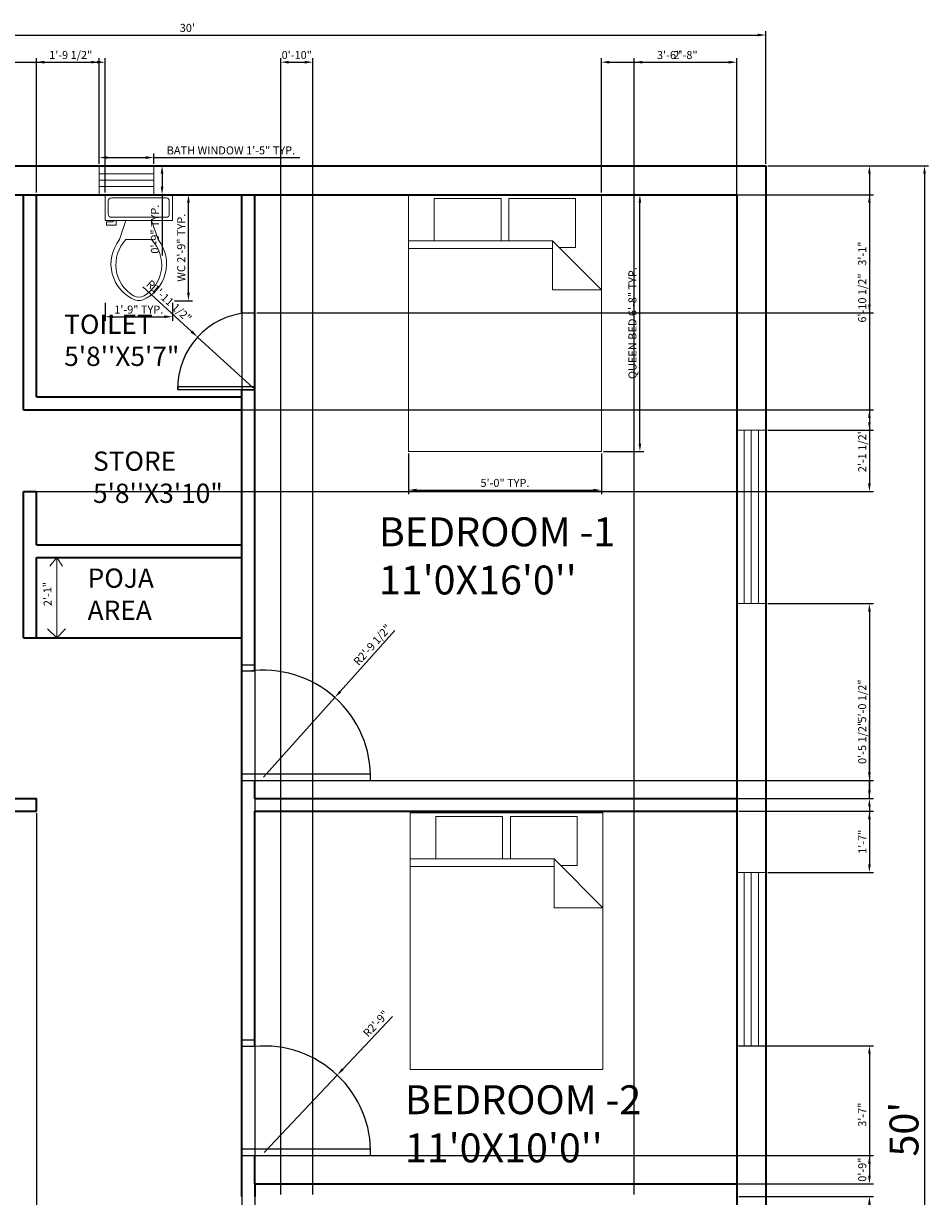
# Model space of a CAD drawing. Units: inches. Extents: x 2572 to 3021, y 1553 to 2232.
# Tile 3 of 3: x 2739 to 3021, y 1866 to 2232. Entities that reach past the tile are written whole.
import ezdxf

# ---------------------------------------------------------------- set-up
doc = ezdxf.new("R2010")
doc.units = ezdxf.units.IN
for name, color, linetype, lineweight in [('A-ANNO-DIMS', 2, 'Continuous', 18), ('A-AREA-IDEN', 7, 'Continuous', 25), ('A-DOOR', 3, 'Continuous', 25), ('A-FLOR-FIXT', 9, 'Continuous', 18), ('A-FURN', 8, 'Continuous', 18), ('A-GLAZ', 4, 'Continuous', 18), ('A-WALL', 7, 'Continuous', 35)]:
    doc.layers.add(name, color=color, linetype=linetype, lineweight=lineweight)
doc.styles.get("Standard").update_dxf_attribs({"font": 'arial.ttf'})
doc.dimstyles.new('ISO-25', dxfattribs={"dimtxt": 2.5, "dimasz": 2.5, "dimexe": 1.25, "dimexo": 0.625, "dimtad": 1, "dimdec": 1, "dimlunit": 3, "dimtxsty": 'Standard', "dimcen": 2.5, "dimadec": 0, "dimazin": 0, "dimtfac": 1, "dimtdec": 1, "dimtmove": 0, "dimatfit": 3, "dimfxl": 1, "dimarcsym": 0})

# ---------------------------------------------------------------- blocks, each defined once
blk = doc.blocks.new('Bed - Queen')
for p, q in [((0, -80.00003), (0, 0)), ((0, 0), (59.99999, 0)), ((59.99999, 0), (59.99999, -80.00003)), ((7.99999, -1.2), (28.79998, -1.2)), ((7.99999, -14.4), (7.99999, -1.2)), ((28.79998, -1.2), (28.79998, -14.4)), ((31.19999, -1.2), (51.99999, -1.2)), ((31.19999, -14.4), (31.19999, -1.2)), ((51.99999, -1.2), (51.99999, -16.4)), ((0, -14.4), (44.8, -14.4)), ((59.99999, -29.6), (44.8, -14.4)), ((44.8, -14.4), (44.8, -29.6)), ((44.8, -16.8), (0, -16.8)), ((51.99999, -16.4), (46.79936, -16.4)), ((44.8, -29.6), (59.99999, -29.6)), ((59.99999, -80.00003), (0, -80.00003))]:
    blk.add_line(p, q)
blk = doc.blocks.new('Toilet - top')
for p, q in [((9.5, -6), (9.5, -2)), ((-10, -8.5), (-8, -8.5)), ((-10, -9.5), (-10, -8.5)), ((-7, -9.5), (-10, -9.5)), ((-8, -8.5), (-8, -8)), ((-7, -8), (-7, -9.5)), ((-4, -8), (-6, -14)), ((4, -8), (6, -14)), ((4, -14), (-4, -14))]:
    blk.add_line(p, q)
blk.add_lwpolyline([(10.5, -8), (10.5, 0), (-10.5, 0), (-10.5, -8)], close=True)
for points in [[(-9.5, -2), (-9.5, -6)], [(8.5, -1), (-8.5, -1)], [(-8.5, -7), (8.5, -7)]]:
    blk.add_lwpolyline(points)
for centre, radius, start, end in [((-8.62, -1.88), 0.884, 81.8699, 188.1301), ((8.62, -1.88), 0.884, 351.8699, 98.1301), ((-8.62, -6.12), 0.884, 171.8699, 278.1301), ((8.62, -6.12), 0.884, 261.8699, 8.1301), ((3.52, -21.58), 12.17, 141.4691, 247.9714), ((4.2, -21.82), 11.33, 136.3677, 238.9468), ((-3.52, -21.58), 12.17, 292.0284, 38.5307), ((-4.2, -21.82), 11.33, 301.053, 43.6321), ((0, -27.88), 4, 245.7318, 294.2682), ((0, -29), 4, 254.8605, 285.1395)]:
    blk.add_arc(centre, radius, start, end)
blk = doc.blocks.new('Window - Wood Frame 36 in. Wide plan')
for p, q in [((0, 6), (0, 0)), ((36, 6), (36, 0)), ((0, 4.5), (36, 4.5)), ((0, 3), (36, 3)), ((0, 1.5), (36, 1.5))]:
    blk.add_line(p, q)
blk = doc.blocks.new('*D6')
at = {"layer": 'A-ANNO-DIMS', "color": 0, "lineweight": -2, "transparency": 16777216}
for p, q in [((2970.8, 2187.37), (3020.83, 2187.37)), ((3019.58, 2184.87), (3019.58, 1589.87)), ((2970.8, 1587.37), (3020.83, 1587.37))]:
    blk.add_line(p, q, dxfattribs=at)
at = {"layer": 'A-ANNO-DIMS', "color": 0, "transparency": 16777216}
for points in [[(3019.16, 2184.87), (3019.99, 2184.87), (3019.58, 2187.37)], [(3019.16, 1589.87), (3019.99, 1589.87), (3019.58, 1587.37)]]:
    blk.add_solid(points, dxfattribs=at)
at = {"layer": 'Defpoints', "color": 0, "transparency": 16777216}
for p in [(2970.18, 2187.37), (2970.18, 1587.37), (3019.58, 1587.37)]:
    blk.add_point(p, dxfattribs=at)
at = {"layer": 'A-ANNO-DIMS', "color": 0, "transparency": 16777216, "insert": (3014.36, 1887.37), "char_height": 9, "attachment_point": 5, "rotation": 90}
blk.add_mtext("50'", dxfattribs=at)
blk = doc.blocks.new('*D7')
at = {"layer": 'A-ANNO-DIMS', "color": 0, "lineweight": -2, "transparency": 16777216}
for p, q in [((2610.18, 2188), (2610.18, 2229.34)), ((2970.18, 2188), (2970.18, 2229.34)), ((2612.68, 2228.09), (2967.68, 2228.09))]:
    blk.add_line(p, q, dxfattribs=at)
at = {"layer": 'A-ANNO-DIMS', "color": 0, "transparency": 16777216}
for points in [[(2612.68, 2228.5), (2612.68, 2227.67), (2610.18, 2228.09)], [(2967.68, 2228.5), (2967.68, 2227.67), (2970.18, 2228.09)]]:
    blk.add_solid(points, dxfattribs=at)
at = {"layer": 'Defpoints', "color": 0, "transparency": 16777216}
for p in [(2970.18, 2228.09), (2610.18, 2187.37), (2970.18, 2187.37)]:
    blk.add_point(p, dxfattribs=at)
at = {"layer": 'A-ANNO-DIMS', "color": 0, "transparency": 16777216, "insert": (2790.18, 2229.99), "char_height": 2.5, "attachment_point": 5}
blk.add_mtext("30'", dxfattribs=at)
blk = doc.blocks.new('WIN-BATH-17IN')
for p, q in [((0, 17), (9, 17)), ((2.5, 17), (2.5, 0)), ((4.5, 17), (4.5, 0)), ((6.5, 17), (6.5, 0)), ((0, 0), (9, 0))]:
    blk.add_line(p, q)
blk = doc.blocks.new('*D12')
at = {"layer": 'A-ANNO-DIMS', "color": 0, "lineweight": -2, "transparency": 16777216}
for p, q in [((2919.63, 2178.37), (2932.26, 2178.37)), ((2931.01, 2100.87), (2931.01, 2175.87)), ((2919.63, 2098.37), (2932.26, 2098.37))]:
    blk.add_line(p, q, dxfattribs=at)
at = {"layer": 'A-ANNO-DIMS', "color": 0, "transparency": 16777216}
for points in [[(2930.59, 2175.87), (2931.42, 2175.87), (2931.01, 2178.37)], [(2930.59, 2100.87), (2931.42, 2100.87), (2931.01, 2098.37)]]:
    blk.add_solid(points, dxfattribs=at)
at = {"layer": 'Defpoints', "color": 0, "transparency": 16777216}
for p in [(2919.01, 2178.37), (2931.01, 2178.37), (2919.01, 2098.37)]:
    blk.add_point(p, dxfattribs=at)
at = {"layer": 'A-ANNO-DIMS', "color": 0, "transparency": 16777216, "insert": (2929.01, 2138.37), "char_height": 2.5, "attachment_point": 5, "rotation": 90}
blk.add_mtext('QUEEN BED 6\'-8" TYP.', dxfattribs=at)
blk = doc.blocks.new('*D13')
at = {"layer": 'A-ANNO-DIMS', "color": 0, "lineweight": -2, "transparency": 16777216}
for p, q in [((2859.01, 2097.75), (2859.01, 2085.12)), ((2919.01, 2097.75), (2919.01, 2085.12)), ((2861.51, 2086.37), (2916.51, 2086.37))]:
    blk.add_line(p, q, dxfattribs=at)
at = {"layer": 'A-ANNO-DIMS', "color": 0, "transparency": 16777216}
for points in [[(2861.51, 2086.79), (2861.51, 2085.96), (2859.01, 2086.37)], [(2916.51, 2086.79), (2916.51, 2085.96), (2919.01, 2086.37)]]:
    blk.add_solid(points, dxfattribs=at)
at = {"layer": 'Defpoints', "color": 0, "transparency": 16777216}
for p in [(2859.01, 2098.37), (2919.01, 2098.37), (2919.01, 2086.37)]:
    blk.add_point(p, dxfattribs=at)
at = {"layer": 'A-ANNO-DIMS', "color": 0, "transparency": 16777216, "insert": (2889.01, 2088.28), "char_height": 2.5, "attachment_point": 5}
blk.add_mtext('5\'-0" TYP.', dxfattribs=at)
blk = doc.blocks.new('*D14')
at = {"layer": 'A-ANNO-DIMS', "color": 0, "lineweight": -2, "transparency": 16777216}
for p, q in [((2786.18, 2178.37), (2791.76, 2178.37)), ((2790.51, 2147.83), (2790.51, 2175.87)), ((2786.18, 2145.33), (2791.76, 2145.33))]:
    blk.add_line(p, q, dxfattribs=at)
at = {"layer": 'A-ANNO-DIMS', "color": 0, "transparency": 16777216}
for points in [[(2790.1, 2175.87), (2790.93, 2175.87), (2790.51, 2178.37)], [(2790.1, 2147.83), (2790.93, 2147.83), (2790.51, 2145.33)]]:
    blk.add_solid(points, dxfattribs=at)
at = {"layer": 'Defpoints', "color": 0, "transparency": 16777216}
for p in [(2785.56, 2178.37), (2790.51, 2178.37), (2785.56, 2145.33)]:
    blk.add_point(p, dxfattribs=at)
at = {"layer": 'A-ANNO-DIMS', "color": 0, "transparency": 16777216, "insert": (2788.59, 2161.85), "char_height": 2.5, "attachment_point": 5, "rotation": 90}
blk.add_mtext('WC 2\'-9" TYP.', dxfattribs=at)
blk = doc.blocks.new('*D15')
at = {"layer": 'A-ANNO-DIMS', "color": 0, "lineweight": -2, "transparency": 16777216}
for p, q in [((2764.56, 2144.7), (2764.56, 2139.12)), ((2785.56, 2144.7), (2785.56, 2139.12)), ((2767.06, 2140.37), (2783.06, 2140.37))]:
    blk.add_line(p, q, dxfattribs=at)
at = {"layer": 'A-ANNO-DIMS', "color": 0, "transparency": 16777216}
for points in [[(2767.06, 2140.79), (2767.06, 2139.95), (2764.56, 2140.37)], [(2783.06, 2140.79), (2783.06, 2139.95), (2785.56, 2140.37)]]:
    blk.add_solid(points, dxfattribs=at)
at = {"layer": 'Defpoints', "color": 0, "transparency": 16777216}
for p in [(2764.56, 2145.33), (2785.56, 2145.33), (2785.56, 2140.37)]:
    blk.add_point(p, dxfattribs=at)
at = {"layer": 'A-ANNO-DIMS', "color": 0, "transparency": 16777216, "insert": (2775.06, 2142.27), "char_height": 2.5, "attachment_point": 5}
blk.add_mtext('1\'-9" TYP.', dxfattribs=at)
blk = doc.blocks.new('*D18')
at = {"layer": 'A-ANNO-DIMS', "color": 0, "lineweight": -2, "transparency": 16777216}
for p, q in [((2762.75, 2188), (2762.75, 2191.17)), ((2765.25, 2189.92), (2777.25, 2189.92)), ((2779.75, 2188), (2779.75, 2191.17)), ((2779.75, 2189.92), (2825.21, 2189.92))]:
    blk.add_line(p, q, dxfattribs=at)
at = {"layer": 'A-ANNO-DIMS', "color": 0, "transparency": 16777216}
for points in [[(2765.25, 2190.34), (2765.25, 2189.51), (2762.75, 2189.92)], [(2777.25, 2190.34), (2777.25, 2189.51), (2779.75, 2189.92)]]:
    blk.add_solid(points, dxfattribs=at)
at = {"layer": 'Defpoints', "color": 0, "transparency": 16777216}
for p in [(2779.75, 2189.92), (2762.75, 2187.37), (2779.75, 2187.37)]:
    blk.add_point(p, dxfattribs=at)
at = {"layer": 'A-ANNO-DIMS', "color": 0, "transparency": 16777216, "insert": (2803.73, 2191.84), "char_height": 2.5, "attachment_point": 5}
blk.add_mtext('BATH WINDOW 1\'-5" TYP.', dxfattribs=at)
blk = doc.blocks.new('*D19')
at = {"layer": 'A-ANNO-DIMS', "color": 0, "lineweight": -2, "transparency": 16777216}
for p, q in [((2780.37, 2187.37), (2783.55, 2187.37)), ((2782.3, 2184.87), (2782.3, 2180.87)), ((2780.37, 2178.37), (2783.55, 2178.37)), ((2782.3, 2178.37), (2782.3, 2159.39))]:
    blk.add_line(p, q, dxfattribs=at)
at = {"layer": 'A-ANNO-DIMS', "color": 0, "transparency": 16777216}
for points in [[(2781.88, 2184.87), (2782.72, 2184.87), (2782.3, 2187.37)], [(2781.88, 2180.87), (2782.72, 2180.87), (2782.3, 2178.37)]]:
    blk.add_solid(points, dxfattribs=at)
at = {"layer": 'Defpoints', "color": 0, "transparency": 16777216}
for p in [(2779.75, 2187.37), (2779.75, 2178.37), (2782.3, 2178.37)]:
    blk.add_point(p, dxfattribs=at)
at = {"layer": 'A-ANNO-DIMS', "color": 0, "transparency": 16777216, "insert": (2780.4, 2167.63), "char_height": 2.5, "attachment_point": 5, "rotation": 90}
blk.add_mtext('0\'-9" TYP.', dxfattribs=at)
blk = doc.blocks.new('*D21')
at = {"layer": 'A-ANNO-DIMS', "color": 0, "lineweight": -2, "transparency": 16777216}
for p, q in [((2699.85, 2188), (2699.85, 2220.88)), ((2702.35, 2219.63), (2760.25, 2219.63)), ((2762.75, 2188), (2762.75, 2220.88))]:
    blk.add_line(p, q, dxfattribs=at)
at = {"layer": 'A-ANNO-DIMS', "color": 0, "transparency": 16777216}
for points in [[(2702.35, 2220.05), (2702.35, 2219.21), (2699.85, 2219.63)], [(2760.25, 2220.05), (2760.25, 2219.21), (2762.75, 2219.63)]]:
    blk.add_solid(points, dxfattribs=at)
at = {"layer": 'Defpoints', "color": 0, "transparency": 16777216}
for p in [(2762.75, 2219.63), (2699.85, 2187.37), (2762.75, 2187.37)]:
    blk.add_point(p, dxfattribs=at)
at = {"layer": 'A-ANNO-DIMS', "color": 0, "transparency": 16777216, "insert": (2731.3, 2221.53), "char_height": 2.5, "attachment_point": 5}
blk.add_mtext('5\'-3"', dxfattribs=at)
blk = doc.blocks.new('*D25')
at = {"layer": 'A-ANNO-DIMS', "color": 0, "lineweight": -2, "transparency": 16777216}
for p, q in [((2970.8, 2187.37), (3003.68, 2187.37)), ((3002.43, 2184.87), (3002.43, 2107.51)), ((2970.8, 2105.01), (3003.68, 2105.01))]:
    blk.add_line(p, q, dxfattribs=at)
at = {"layer": 'A-ANNO-DIMS', "color": 0, "transparency": 16777216}
for points in [[(3002.02, 2184.87), (3002.85, 2184.87), (3002.43, 2187.37)], [(3002.02, 2107.51), (3002.85, 2107.51), (3002.43, 2105.01)]]:
    blk.add_solid(points, dxfattribs=at)
at = {"layer": 'Defpoints', "color": 0, "transparency": 16777216}
for p in [(2970.18, 2187.37), (2970.18, 2105.01), (3002.43, 2105.01)]:
    blk.add_point(p, dxfattribs=at)
at = {"layer": 'A-ANNO-DIMS', "color": 0, "transparency": 16777216, "insert": (3000.51, 2146.19), "char_height": 2.5, "attachment_point": 5, "rotation": 90}
blk.add_mtext('6\'-10 1/2"', dxfattribs=at)
blk = doc.blocks.new('*D26')
at = {"layer": 'A-ANNO-DIMS', "color": 0, "lineweight": -2, "transparency": 16777216}
for p, q in [((2970.8, 2051.01), (3003.68, 2051.01)), ((3002.43, 2048.51), (3002.43, 1992.87)), ((2961.8, 1990.37), (3003.68, 1990.37))]:
    blk.add_line(p, q, dxfattribs=at)
at = {"layer": 'A-ANNO-DIMS', "color": 0, "transparency": 16777216}
for points in [[(3002.02, 2048.51), (3002.85, 2048.51), (3002.43, 2051.01)], [(3002.02, 1992.87), (3002.85, 1992.87), (3002.43, 1990.37)]]:
    blk.add_solid(points, dxfattribs=at)
at = {"layer": 'Defpoints', "color": 0, "transparency": 16777216}
for p in [(2970.18, 2051.01), (2961.18, 1990.37), (3002.43, 1990.37)]:
    blk.add_point(p, dxfattribs=at)
at = {"layer": 'A-ANNO-DIMS', "color": 0, "transparency": 16777216, "insert": (3000.51, 2020.69), "char_height": 2.5, "attachment_point": 5, "rotation": 90}
blk.add_mtext('5\'-0 1/2"', dxfattribs=at)
blk = doc.blocks.new('*D27')
at = {"layer": 'A-ANNO-DIMS', "color": 0, "lineweight": -2, "transparency": 16777216}
for p, q in [((2961.8, 1986.37), (3003.68, 1986.37)), ((3002.43, 1983.87), (3002.43, 1969.83)), ((2970.8, 1967.33), (3003.68, 1967.33))]:
    blk.add_line(p, q, dxfattribs=at)
at = {"layer": 'A-ANNO-DIMS', "color": 0, "transparency": 16777216}
for points in [[(3002.02, 1983.87), (3002.85, 1983.87), (3002.43, 1986.37)], [(3002.02, 1969.83), (3002.85, 1969.83), (3002.43, 1967.33)]]:
    blk.add_solid(points, dxfattribs=at)
at = {"layer": 'Defpoints', "color": 0, "transparency": 16777216}
for p in [(2961.18, 1986.37), (2970.18, 1967.33), (3002.43, 1967.33)]:
    blk.add_point(p, dxfattribs=at)
at = {"layer": 'A-ANNO-DIMS', "color": 0, "transparency": 16777216, "insert": (3000.55, 1976.85), "char_height": 2.5, "attachment_point": 5, "rotation": 90}
blk.add_mtext('1\'-7"', dxfattribs=at)
blk = doc.blocks.new('*D28')
at = {"layer": 'A-ANNO-DIMS', "color": 0, "lineweight": -2, "transparency": 16777216}
for p, q in [((2961.8, 1866.37), (3003.68, 1866.37)), ((3002.43, 1863.87), (3002.43, 1861)), ((2970.8, 1858.5), (3003.68, 1858.5)), ((3002.43, 1858.5), (3002.43, 1848.1))]:
    blk.add_line(p, q, dxfattribs=at)
at = {"layer": 'A-ANNO-DIMS', "color": 0, "transparency": 16777216}
for points in [[(3002.02, 1863.87), (3002.85, 1863.87), (3002.43, 1866.37)], [(3002.02, 1861), (3002.85, 1861), (3002.43, 1858.5)]]:
    blk.add_solid(points, dxfattribs=at)
at = {"layer": 'Defpoints', "color": 0, "transparency": 16777216}
for p in [(2961.18, 1866.37), (2970.18, 1858.5), (3002.43, 1858.5)]:
    blk.add_point(p, dxfattribs=at)
at = {"layer": 'A-ANNO-DIMS', "color": 0, "transparency": 16777216, "insert": (3000.53, 1852.05), "char_height": 2.5, "attachment_point": 5, "rotation": 90}
blk.add_mtext('0\'-8"', dxfattribs=at)
blk = doc.blocks.new('*D30')
at = {"layer": 'A-ANNO-DIMS', "color": 0, "lineweight": -2, "transparency": 16777216}
for p, q in [((2819.22, 1867), (2819.22, 2220.88)), ((2821.72, 2219.63), (2826.72, 2219.63)), ((2829.22, 1867), (2829.22, 2220.88))]:
    blk.add_line(p, q, dxfattribs=at)
at = {"layer": 'A-ANNO-DIMS', "color": 0, "transparency": 16777216}
for points in [[(2821.72, 2220.05), (2821.72, 2219.21), (2819.22, 2219.63)], [(2826.72, 2220.05), (2826.72, 2219.21), (2829.22, 2219.63)]]:
    blk.add_solid(points, dxfattribs=at)
at = {"layer": 'Defpoints', "color": 0, "transparency": 16777216}
for p in [(2829.22, 2219.63), (2819.22, 1866.37), (2829.22, 1866.37)]:
    blk.add_point(p, dxfattribs=at)
at = {"layer": 'A-ANNO-DIMS', "color": 0, "transparency": 16777216, "insert": (2824.22, 2221.53), "char_height": 2.5, "attachment_point": 5}
blk.add_mtext('0\'-10"', dxfattribs=at)
blk = doc.blocks.new('*D31')
at = {"layer": 'A-ANNO-DIMS', "color": 0, "lineweight": -2, "transparency": 16777216}
for p, q in [((2929.22, 1867), (2929.22, 2220.88)), ((2931.72, 2219.63), (2958.68, 2219.63)), ((2961.18, 1867), (2961.18, 2220.88))]:
    blk.add_line(p, q, dxfattribs=at)
at = {"layer": 'A-ANNO-DIMS', "color": 0, "transparency": 16777216}
for points in [[(2931.72, 2220.05), (2931.72, 2219.21), (2929.22, 2219.63)], [(2958.68, 2220.05), (2958.68, 2219.21), (2961.18, 2219.63)]]:
    blk.add_solid(points, dxfattribs=at)
at = {"layer": 'Defpoints', "color": 0, "transparency": 16777216}
for p in [(2961.18, 2219.63), (2929.22, 1866.37), (2961.18, 1866.37)]:
    blk.add_point(p, dxfattribs=at)
at = {"layer": 'A-ANNO-DIMS', "color": 0, "transparency": 16777216, "insert": (2945.2, 2221.53), "char_height": 2.5, "attachment_point": 5}
blk.add_mtext('2\'-8"', dxfattribs=at)
blk = doc.blocks.new('*D32')
at = {"layer": 'A-ANNO-DIMS', "color": 0, "lineweight": -2, "transparency": 16777216}
for p, q in [((2743.18, 2179), (2743.18, 2220.88)), ((2745.68, 2219.63), (2762.06, 2219.63)), ((2764.56, 2179), (2764.56, 2220.88))]:
    blk.add_line(p, q, dxfattribs=at)
at = {"layer": 'A-ANNO-DIMS', "color": 0, "transparency": 16777216}
for points in [[(2745.68, 2220.05), (2745.68, 2219.21), (2743.18, 2219.63)], [(2762.06, 2220.05), (2762.06, 2219.21), (2764.56, 2219.63)]]:
    blk.add_solid(points, dxfattribs=at)
at = {"layer": 'Defpoints', "color": 0, "transparency": 16777216}
for p in [(2764.56, 2219.63), (2743.18, 2178.37), (2764.56, 2178.37)]:
    blk.add_point(p, dxfattribs=at)
at = {"layer": 'A-ANNO-DIMS', "color": 0, "transparency": 16777216, "insert": (2753.87, 2221.55), "char_height": 2.5, "attachment_point": 5}
blk.add_mtext('1\'-9 1/2"', dxfattribs=at)
blk = doc.blocks.new('*D33')
at = {"layer": 'A-ANNO-DIMS', "color": 0, "lineweight": -2, "transparency": 16777216}
for p, q in [((2811.8, 2178.37), (3003.68, 2178.37)), ((3002.43, 2175.87), (3002.43, 2144.12)), ((2811.8, 2141.62), (3003.68, 2141.62))]:
    blk.add_line(p, q, dxfattribs=at)
at = {"layer": 'A-ANNO-DIMS', "color": 0, "transparency": 16777216}
for points in [[(3002.02, 2175.87), (3002.85, 2175.87), (3002.43, 2178.37)], [(3002.02, 2144.12), (3002.85, 2144.12), (3002.43, 2141.62)]]:
    blk.add_solid(points, dxfattribs=at)
at = {"layer": 'Defpoints', "color": 0, "transparency": 16777216}
for p in [(2811.18, 2178.37), (2811.18, 2141.62), (3002.43, 2141.62)]:
    blk.add_point(p, dxfattribs=at)
at = {"layer": 'A-ANNO-DIMS', "color": 0, "transparency": 16777216, "insert": (3000.53, 2160), "char_height": 2.5, "attachment_point": 5, "rotation": 90}
blk.add_mtext('3\'-1"', dxfattribs=at)
blk = doc.blocks.new('*D34')
at = {"layer": 'A-ANNO-DIMS', "color": 0, "lineweight": -2, "transparency": 16777216}
for p, q in [((2739.8, 2111.37), (3003.68, 2111.37)), ((3002.43, 2108.87), (3002.43, 2088.44)), ((2739.8, 2085.94), (3003.68, 2085.94))]:
    blk.add_line(p, q, dxfattribs=at)
at = {"layer": 'A-ANNO-DIMS', "color": 0, "transparency": 16777216}
for points in [[(3002.02, 2108.87), (3002.85, 2108.87), (3002.43, 2111.37)], [(3002.02, 2088.44), (3002.85, 2088.44), (3002.43, 2085.94)]]:
    blk.add_solid(points, dxfattribs=at)
at = {"layer": 'Defpoints', "color": 0, "transparency": 16777216}
for p in [(2739.18, 2111.37), (2739.18, 2085.94), (3002.43, 2085.94)]:
    blk.add_point(p, dxfattribs=at)
at = {"layer": 'A-ANNO-DIMS', "color": 0, "transparency": 16777216, "insert": (3000.51, 2098.66), "char_height": 2.5, "attachment_point": 5, "rotation": 90}
blk.add_mtext('2\'-1 1/2"', dxfattribs=at)
blk = doc.blocks.new('*D35')
at = {"layer": 'A-ANNO-DIMS', "color": 0, "lineweight": -2, "transparency": 16777216}
for p, q in [((2807.18, 1995.31), (2807.18, 1553.87)), ((2743.18, 1985.75), (2743.18, 1553.87)), ((2745.68, 1555.12), (2804.68, 1555.12))]:
    blk.add_line(p, q, dxfattribs=at)
at = {"layer": 'A-ANNO-DIMS', "color": 0, "transparency": 16777216}
for points in [[(2745.68, 1555.54), (2745.68, 1554.7), (2743.18, 1555.12)], [(2804.68, 1555.54), (2804.68, 1554.7), (2807.18, 1555.12)]]:
    blk.add_solid(points, dxfattribs=at)
at = {"layer": 'Defpoints', "color": 0, "transparency": 16777216}
for p in [(2807.18, 1995.94), (2743.18, 1986.37), (2807.18, 1555.12)]:
    blk.add_point(p, dxfattribs=at)
at = {"layer": 'A-ANNO-DIMS', "color": 0, "transparency": 16777216, "insert": (2775.18, 1557.02), "char_height": 2.5, "attachment_point": 5}
blk.add_mtext('5\'-4"', dxfattribs=at)
blk = doc.blocks.new('*D37')
at = {"layer": 'A-ANNO-DIMS', "color": 0, "lineweight": -2, "transparency": 16777216}
for p, q in [((3002.43, 1998.44), (3002.43, 2014.66)), ((2811.8, 1995.94), (3003.68, 1995.94)), ((3002.43, 1990.37), (3002.43, 1995.94)), ((2811.8, 1990.37), (3003.68, 1990.37)), ((3002.43, 1987.87), (3002.43, 1985.37))]:
    blk.add_line(p, q, dxfattribs=at)
at = {"layer": 'A-ANNO-DIMS', "color": 0, "transparency": 16777216}
for points in [[(3002.02, 1998.44), (3002.85, 1998.44), (3002.43, 1995.94)], [(3002.02, 1987.87), (3002.85, 1987.87), (3002.43, 1990.37)]]:
    blk.add_solid(points, dxfattribs=at)
at = {"layer": 'Defpoints', "color": 0, "transparency": 16777216}
for p in [(2811.18, 1995.94), (3002.43, 1995.94), (2811.18, 1990.37)]:
    blk.add_point(p, dxfattribs=at)
at = {"layer": 'A-ANNO-DIMS', "color": 0, "transparency": 16777216, "insert": (3000.51, 2007.8), "char_height": 2.5, "attachment_point": 5, "rotation": 90}
blk.add_mtext('0\'-5 1/2"', dxfattribs=at)
blk = doc.blocks.new('*D39')
at = {"layer": 'A-ANNO-DIMS', "color": 0, "lineweight": -2, "transparency": 16777216}
for p, q in [((2807.18, 2177.75), (2807.18, 1553.87)), ((2811.18, 2177.75), (2811.18, 1553.87)), ((2804.68, 1555.12), (2802.18, 1555.12)), ((2807.18, 1555.12), (2811.18, 1555.12)), ((2813.68, 1555.12), (2824.07, 1555.12))]:
    blk.add_line(p, q, dxfattribs=at)
at = {"layer": 'A-ANNO-DIMS', "color": 0, "transparency": 16777216}
for points in [[(2804.68, 1555.54), (2804.68, 1554.7), (2807.18, 1555.12)], [(2813.68, 1555.54), (2813.68, 1554.7), (2811.18, 1555.12)]]:
    blk.add_solid(points, dxfattribs=at)
at = {"layer": 'Defpoints', "color": 0, "transparency": 16777216}
for p in [(2807.18, 2178.37), (2811.18, 2178.37), (2811.18, 1555.12)]:
    blk.add_point(p, dxfattribs=at)
at = {"layer": 'A-ANNO-DIMS', "color": 0, "transparency": 16777216, "insert": (2820.12, 1557.02), "char_height": 2.5, "attachment_point": 5}
blk.add_mtext('0\'-4"', dxfattribs=at)
blk = doc.blocks.new('*D43')
at = {"layer": 'A-ANNO-DIMS', "color": 0, "lineweight": -2, "transparency": 16777216}
for p, q in [((2919.01, 2179), (2919.01, 2220.88)), ((2921.51, 2219.63), (2958.68, 2219.63)), ((2961.18, 2179), (2961.18, 2220.88))]:
    blk.add_line(p, q, dxfattribs=at)
at = {"layer": 'A-ANNO-DIMS', "color": 0, "transparency": 16777216}
for points in [[(2921.51, 2220.05), (2921.51, 2219.21), (2919.01, 2219.63)], [(2958.68, 2220.05), (2958.68, 2219.21), (2961.18, 2219.63)]]:
    blk.add_solid(points, dxfattribs=at)
at = {"layer": 'Defpoints', "color": 0, "transparency": 16777216}
for p in [(2961.18, 2219.63), (2919.01, 2178.37), (2961.18, 2178.37)]:
    blk.add_point(p, dxfattribs=at)
at = {"layer": 'A-ANNO-DIMS', "color": 0, "transparency": 16777216, "insert": (2940.09, 2221.53), "char_height": 2.5, "attachment_point": 5}
blk.add_mtext('3\'-6"', dxfattribs=at)
blk = doc.blocks.new('*D44')
at = {"layer": 'A-ANNO-DIMS', "color": 0, "lineweight": -2, "transparency": 16777216}
for p, q in [((2961.8, 1913.33), (3003.68, 1913.33)), ((3002.43, 1910.83), (3002.43, 1872.87)), ((2961.8, 1870.37), (3003.68, 1870.37))]:
    blk.add_line(p, q, dxfattribs=at)
at = {"layer": 'A-ANNO-DIMS', "color": 0, "transparency": 16777216}
for points in [[(3002.02, 1910.83), (3002.85, 1910.83), (3002.43, 1913.33)], [(3002.02, 1872.87), (3002.85, 1872.87), (3002.43, 1870.37)]]:
    blk.add_solid(points, dxfattribs=at)
at = {"layer": 'Defpoints', "color": 0, "transparency": 16777216}
for p in [(2961.18, 1913.33), (2961.18, 1870.37), (3002.43, 1870.37)]:
    blk.add_point(p, dxfattribs=at)
at = {"layer": 'A-ANNO-DIMS', "color": 0, "transparency": 16777216, "insert": (3000.53, 1891.85), "char_height": 2.5, "attachment_point": 5, "rotation": 90}
blk.add_mtext('3\'-7"', dxfattribs=at)
blk = doc.blocks.new('*D45')
at = {"layer": 'A-ANNO-DIMS', "color": 0, "lineweight": -2, "transparency": 16777216}
for p, q in [((2811.8, 1879.13), (3003.68, 1879.13)), ((3002.43, 1876.63), (3002.43, 1872.87)), ((2811.8, 1870.37), (3003.68, 1870.37))]:
    blk.add_line(p, q, dxfattribs=at)
at = {"layer": 'A-ANNO-DIMS', "color": 0, "transparency": 16777216}
for points in [[(3002.02, 1876.63), (3002.85, 1876.63), (3002.43, 1879.13)], [(3002.02, 1872.87), (3002.85, 1872.87), (3002.43, 1870.37)]]:
    blk.add_solid(points, dxfattribs=at)
at = {"layer": 'Defpoints', "color": 0, "transparency": 16777216}
for p in [(2811.18, 1879.13), (2811.18, 1870.37), (3002.43, 1870.37)]:
    blk.add_point(p, dxfattribs=at)
at = {"layer": 'A-ANNO-DIMS', "color": 0, "transparency": 16777216, "insert": (3000.53, 1874.75), "char_height": 2.5, "attachment_point": 5, "rotation": 90}
blk.add_mtext('0\'-9"', dxfattribs=at)
blk = doc.blocks.new('*D48')
at = {"layer": 'A-ANNO-DIMS', "color": 0, "lineweight": -2, "transparency": 16777216}
for p, q in [((2854.79, 2042.69), (2837.75, 2023.64)), ((2813.86, 1996.94), (2836.09, 2021.78))]:
    blk.add_line(p, q, dxfattribs=at)
at = {"layer": 'A-ANNO-DIMS', "color": 0, "transparency": 16777216}
blk.add_solid([(2837.44, 2023.92), (2838.06, 2023.36), (2836.09, 2021.78)], dxfattribs=at)
at = {"layer": 'Defpoints', "color": 0, "transparency": 16777216}
for p in [(2836.09, 2021.78), (2813.86, 1996.94)]:
    blk.add_point(p, dxfattribs=at)
at = {"layer": 'A-ANNO-DIMS', "color": 0, "transparency": 16777216, "insert": (2847.99, 2037.96), "char_height": 2.5, "attachment_point": 5, "rotation": 48.1792}
blk.add_mtext('R2\'-9 1/2"', dxfattribs=at)
blk = doc.blocks.new('*D49')
at = {"layer": 'A-ANNO-DIMS', "color": 0, "lineweight": -2, "transparency": 16777216}
for p, q in [((2853.99, 1922.41), (2838.53, 1906.03)), ((2814.07, 1880.13), (2836.81, 1904.22))]:
    blk.add_line(p, q, dxfattribs=at)
at = {"layer": 'A-ANNO-DIMS', "color": 0, "transparency": 16777216}
blk.add_solid([(2838.22, 1906.32), (2838.83, 1905.75), (2836.81, 1904.22)], dxfattribs=at)
at = {"layer": 'Defpoints', "color": 0, "transparency": 16777216}
for p in [(2836.81, 1904.22), (2814.07, 1880.13)]:
    blk.add_point(p, dxfattribs=at)
at = {"layer": 'A-ANNO-DIMS', "color": 0, "transparency": 16777216, "insert": (2849.08, 1919.97), "char_height": 2.5, "attachment_point": 5, "rotation": 46.6361}
blk.add_mtext('R2\'-9"', dxfattribs=at)
blk = doc.blocks.new('*D50')
at = {"layer": 'A-ANNO-DIMS', "color": 0, "lineweight": -2, "transparency": 16777216}
for p, q in [((2776.29, 2149.68), (2791.51, 2135.73)), ((2810.71, 2118.13), (2793.36, 2134.04))]:
    blk.add_line(p, q, dxfattribs=at)
at = {"layer": 'A-ANNO-DIMS', "color": 0, "transparency": 16777216}
blk.add_solid([(2791.8, 2136.03), (2791.23, 2135.42), (2793.36, 2134.04)], dxfattribs=at)
at = {"layer": 'Defpoints', "color": 0, "transparency": 16777216}
for p in [(2793.36, 2134.04), (2810.71, 2118.13)]:
    blk.add_point(p, dxfattribs=at)
at = {"layer": 'A-ANNO-DIMS', "color": 0, "transparency": 16777216, "insert": (2784.24, 2145), "char_height": 2.5, "attachment_point": 5, "rotation": 317.4902}
blk.add_mtext('R1\'-11 1/2"', dxfattribs=at)

msp = doc.modelspace()

# ---------------------------------------------------------------- linework, layer by layer
at = {"layer": 'A-ANNO-DIMS'}
for p, q in [((2749.55, 2065.37), (2747.43, 2062.68)), ((2749.55, 2065.37), (2749.55, 2040.37)), ((2749.55, 2065.37), (2751.33, 2062.68)), ((2749.55, 2040.37), (2746.69, 2043.18)), ((2749.55, 2040.37), (2752.3, 2043.18))]:
    msp.add_line(p, q, dxfattribs=at)
at = {"layer": 'A-DOOR'}
for p, q in [((2807.18, 2141.62), (2811.18, 2141.62)), ((2787.17, 2117.62), (2787.17, 2118.62)), ((2787.17, 2118.62), (2811.25, 2118.62)), ((2811.17, 2117.62), (2787.17, 2117.62)), ((2807.18, 2117.62), (2811.18, 2117.62)), ((2807.18, 2031.94), (2811.18, 2031.94)), ((2811.18, 2029.94), (2807.18, 2029.94)), ((2847.18, 1997.94), (2807.18, 1997.94)), ((2807.18, 1995.94), (2811.18, 1995.94)), ((2811.18, 1995.94), (2847.18, 1995.94)), ((2847.18, 1995.94), (2847.18, 1997.94)), ((2807.18, 1915.13), (2811.18, 1915.13)), ((2811.18, 1913.13), (2807.18, 1913.13)), ((2847.18, 1881.13), (2807.18, 1881.13)), ((2807.18, 1879.13), (2811.18, 1879.13)), ((2811.18, 1879.13), (2847.18, 1879.13)), ((2847.18, 1879.13), (2847.18, 1881.13))]:
    msp.add_line(p, q, dxfattribs=at)
for centre, radius, start, end in [((2810.71, 2118.13), 23.54, 93.7369, 181.2417), ((2813.86, 1996.94), 33.33, 358.2807, 98.0789), ((2814.07, 1880.13), 33.13, 358.2701, 95.003)]:
    msp.add_arc(centre, radius, start, end, dxfattribs=at)
at = {"layer": 'A-WALL'}
for p, q in [((2610.18, 2187.37), (2970.18, 2187.37)), ((2970.18, 2187.37), (2970.18, 1587.37)), ((2619.18, 2178.37), (2961.18, 2178.37)), ((2739.18, 2111.37), (2739.18, 2178.37)), ((2739.18, 2111.37), (2739.18, 2178.37)), ((2743.18, 2115.37), (2743.18, 2178.37)), ((2743.18, 2115.37), (2743.18, 2178.37)), ((2807.18, 2141.62), (2807.18, 2178.37)), ((2811.18, 2029.94), (2811.18, 2178.37)), ((2961.18, 2178.37), (2961.18, 1596.37)), ((2743.18, 2115.37), (2807.18, 2115.37)), ((2807.18, 1866.37), (2807.18, 2117.62)), ((2739.18, 2111.37), (2807.18, 2111.37)), ((2739.18, 2040.37), (2739.18, 2085.94)), ((2739.18, 2085.94), (2743.18, 2085.94)), ((2743.18, 2069.37), (2743.18, 2085.94)), ((2743.18, 2069.37), (2807.18, 2069.37)), ((2743.18, 2065.37), (2807.18, 2065.37)), ((2743.18, 2040.37), (2743.18, 2065.37)), ((2739.18, 2040.37), (2807.18, 2040.37)), ((2811.18, 1990.37), (2811.18, 1995.94)), ((2619.18, 1990.37), (2743.18, 1990.37)), ((2743.18, 1986.37), (2743.18, 1990.37)), ((2743.18, 1986.37), (2743.18, 1990.37)), ((2811.18, 1990.37), (2961.18, 1990.37)), ((2619.18, 1986.37), (2743.18, 1986.37)), ((2811.18, 1913.13), (2811.18, 1986.37)), ((2811.18, 1986.37), (2961.18, 1986.37)), ((2811.18, 1870.37), (2811.18, 1879.13)), ((2811.18, 1870.37), (2961.18, 1870.37)), ((2811.18, 1870.37), (2811.18, 1866.37))]:
    msp.add_line(p, q, dxfattribs=at)

# ---------------------------------------------------------------- block references
at = {"layer": 'A-FLOR-FIXT'}
msp.add_blockref('Toilet - top', (2775.06, 2178.37), dxfattribs=at)
at = {"layer": 'A-FURN'}
for p in [(2859.01, 2178.37), (2859.49, 1985.91)]:
    msp.add_blockref('Bed - Queen', p, dxfattribs=at)
at = {"layer": 'A-GLAZ', "rotation": 269.9999999999973}
msp.add_blockref('WIN-BATH-17IN', (2762.75, 2187.37), dxfattribs=at)
at = {"layer": 'A-GLAZ', "xscale": 1.5, "yscale": 1.5, "zscale": 1.5, "rotation": 90}
for p in [(2970.18, 2051.01), (2970.18, 1913.33)]:
    msp.add_blockref('Window - Wood Frame 36 in. Wide plan', p, dxfattribs=at)

# ---------------------------------------------------------------- texts
at = {"layer": 'A-ANNO-DIMS', "insert": (2745.45, 2050.21), "char_height": 2.5, "attachment_point": 1, "rotation": 91.1222}
msp.add_mtext('2\'-1"', dxfattribs=at)
at = {"layer": 'A-AREA-IDEN', "attachment_point": 1}
for s, width, insert, char_height in [('TOILET\\P5\'8\'\'X5\'7"', 2.3965, (2751.84, 2141.03), 6), ('STORE\\P5\'8\'\'X3\'10"', 6, (2760.82, 2098.38), 6), ("\\pxt12;BEDROOM -1                     \\P\\ptz;11'0X16'0''", 94.3643, (2849.77, 2077.88), 9), ('POJA AREA', 2.3965, (2759.14, 2061.95), 6), ("\\pxt12;BEDROOM -2                     \\P\\ptz;11'0X10'0''", 94.3643, (2857.86, 1901.02), 9)]:
    msp.add_mtext_dynamic_manual_height_columns(s, width=width, gutter_width=12.5, heights=[0], dxfattribs=dict(at, insert=insert, char_height=char_height))

# ---------------------------------------------------------------- dimensions: what is measured, and where the dimension line sits
at = {"layer": 'A-ANNO-DIMS'}
for base, p1, p2, override, picture, middle in [((2970.18, 2228.09), (2610.18, 2187.37), (2970.18, 2187.37), {"dimclrd": 0, "dimclre": 0, "dimclrt": 0}, '*D7', (2790.18, 2229.99)), ((2764.56, 2219.63), (2743.18, 2178.37), (2764.56, 2178.37), {"dimdec": 1, "dimlfac": 1, "dimrnd": 0, "dimzin": 1, "dimdsep": 46, "dimlunit": 4, "dimfrac": 2}, '*D32', (2753.87, 2221.55)), ((2762.75, 2219.63), (2699.85, 2187.37), (2762.75, 2187.37), {"dimdec": 1, "dimlfac": 1, "dimrnd": 0, "dimzin": 1, "dimdsep": 46, "dimlunit": 4, "dimfrac": 2}, '*D21', (2731.3, 2221.53)), ((2829.22, 2219.63), (2819.22, 1866.37), (2829.22, 1866.37), {"dimdec": 1, "dimlfac": 1, "dimrnd": 0, "dimzin": 1, "dimdsep": 46, "dimlunit": 4, "dimfrac": 2}, '*D30', (2824.22, 2221.53)), ((2961.18, 2219.63), (2919.01, 2178.37), (2961.18, 2178.37), {"dimdec": 1, "dimlfac": 1, "dimrnd": 0, "dimzin": 1, "dimdsep": 46, "dimlunit": 4, "dimfrac": 2}, '*D43', (2940.09, 2221.53)), ((2961.18, 2219.63), (2929.22, 1866.37), (2961.18, 1866.37), {"dimdec": 1, "dimlfac": 1, "dimrnd": 0, "dimzin": 1, "dimdsep": 46, "dimlunit": 4, "dimfrac": 2}, '*D31', (2945.2, 2221.53)), ((2811.18, 1555.12), (2807.18, 2178.37), (2811.18, 2178.37), {"dimdec": 1, "dimlfac": 1, "dimrnd": 0, "dimzin": 1, "dimdsep": 46, "dimlunit": 4, "dimfrac": 2}, '*D39', (2820.12, 1557.02)), ((2807.18, 1555.12), (2743.18, 1986.37), (2807.18, 1995.94), {"dimdec": 1, "dimlfac": 1, "dimrnd": 0, "dimzin": 1, "dimdsep": 46, "dimlunit": 4, "dimfrac": 2}, '*D35', (2775.18, 1557.02))]:
    dim = msp.add_linear_dim(base=base, p1=p1, p2=p2, dimstyle='ISO-25', override=override, dxfattribs=at)
    dim.commit()
    dim.dimension.update_dxf_attribs({"geometry": picture, "text_midpoint": middle})
for base, p1, p2, text, picture, middle in [((2779.75, 2189.92), (2762.75, 2187.37), (2779.75, 2187.37), 'BATH WINDOW <> TYP.', '*D18', (2803.73, 2191.84)), ((2785.56, 2140.37), (2764.56, 2145.33), (2785.56, 2145.33), '<> TYP.', '*D15', (2775.06, 2142.27)), ((2919.01, 2086.37), (2859.01, 2098.37), (2919.01, 2098.37), '<> TYP.', '*D13', (2889.01, 2088.28))]:
    dim = msp.add_linear_dim(base=base, p1=p1, p2=p2, text=text, dimstyle='ISO-25', override={"dimdec": 1, "dimlfac": 1, "dimrnd": 0, "dimzin": 1, "dimdsep": 46, "dimlunit": 4, "dimfrac": 2}, dxfattribs=at)
    dim.commit()
    dim.dimension.update_dxf_attribs({"geometry": picture, "text_midpoint": middle})
for base, p1, p2, angle, text, picture, middle in [((2782.3, 2178.37), (2779.75, 2187.37), (2779.75, 2178.37), 270, '<> TYP.', '*D19', (2780.4, 2167.63)), ((2790.51, 2178.37), (2785.56, 2145.33), (2785.56, 2178.37), 90, 'WC <> TYP.', '*D14', (2788.59, 2161.85)), ((2931.01, 2178.37), (2919.01, 2098.37), (2919.01, 2178.37), 90, 'QUEEN BED <> TYP.', '*D12', (2929.01, 2138.37))]:
    dim = msp.add_linear_dim(base=base, p1=p1, p2=p2, angle=angle, text=text, dimstyle='ISO-25', override={"dimdec": 1, "dimlfac": 1, "dimrnd": 0, "dimzin": 1, "dimdsep": 46, "dimlunit": 4, "dimfrac": 2}, dxfattribs=at)
    dim.commit()
    dim.dimension.update_dxf_attribs({"geometry": picture, "text_midpoint": middle})
for base, p1, p2, override, picture, middle in [((3019.58, 1587.37), (2970.18, 2187.37), (2970.18, 1587.37), {"dimtxt": 9, "dimclrd": 0, "dimclre": 0, "dimclrt": 0}, '*D6', (3014.36, 1887.37)), ((3002.43, 2105.01), (2970.18, 2187.37), (2970.18, 2105.01), {"dimdec": 1, "dimlfac": 1, "dimrnd": 0, "dimzin": 1, "dimdsep": 46, "dimlunit": 4, "dimfrac": 2}, '*D25', (3000.51, 2146.19)), ((3002.4317, 2141.6219), (2811.1767, 2178.3739), (2811.1767, 2141.6219), {"dimdec": 1, "dimlfac": 1, "dimrnd": 0, "dimzin": 1, "dimdsep": 46, "dimlunit": 4, "dimfrac": 2}, '*D33', (3000.5294, 2159.9979)), ((3002.43, 2085.94), (2739.18, 2111.37), (2739.18, 2085.94), {"dimdec": 1, "dimlfac": 1, "dimrnd": 0, "dimzin": 1, "dimdsep": 46, "dimlunit": 4, "dimfrac": 2}, '*D34', (3000.51, 2098.66)), ((3002.43, 1990.37), (2970.18, 2051.01), (2961.18, 1990.37), {"dimdec": 1, "dimlfac": 1, "dimrnd": 0, "dimzin": 1, "dimdsep": 46, "dimlunit": 4, "dimfrac": 2}, '*D26', (3000.51, 2020.69)), ((3002.43, 1995.94), (2811.18, 1990.37), (2811.18, 1995.94), {"dimdec": 1, "dimlfac": 1, "dimrnd": 0, "dimzin": 1, "dimdsep": 46, "dimlunit": 4, "dimfrac": 2}, '*D37', (3000.51, 2007.8)), ((3002.43, 1967.33), (2961.18, 1986.37), (2970.18, 1967.33), {"dimdec": 1, "dimlfac": 1, "dimrnd": 0, "dimzin": 1, "dimdsep": 46, "dimlunit": 4, "dimfrac": 2}, '*D27', (3000.55, 1976.85)), ((3002.43, 1870.37), (2961.18, 1913.33), (2961.18, 1870.37), {"dimdec": 1, "dimlfac": 1, "dimrnd": 0, "dimzin": 1, "dimdsep": 46, "dimlunit": 4, "dimfrac": 2}, '*D44', (3000.53, 1891.85)), ((3002.43, 1870.37), (2811.18, 1879.13), (2811.18, 1870.37), {"dimdec": 1, "dimlfac": 1, "dimrnd": 0, "dimzin": 1, "dimdsep": 46, "dimlunit": 4, "dimfrac": 2}, '*D45', (3000.53, 1874.75)), ((3002.43, 1858.5), (2961.18, 1866.37), (2970.18, 1858.5), {"dimdec": 1, "dimlfac": 1, "dimrnd": 0, "dimzin": 1, "dimdsep": 46, "dimlunit": 4, "dimfrac": 2}, '*D28', (3000.53, 1852.05))]:
    dim = msp.add_linear_dim(base=base, p1=p1, p2=p2, angle=90, dimstyle='ISO-25', override=override, dxfattribs=at)
    dim.commit()
    dim.dimension.update_dxf_attribs({"geometry": picture, "text_midpoint": middle})
for center, mpoint, picture, middle in [((2810.71, 2118.13), (2793.36, 2134.04), '*D50', (2782.94, 2143.58)), ((2813.86, 1996.94), (2836.09, 2021.78), '*D48', (2849.42, 2036.68)), ((2814.07, 1880.13), (2836.81, 1904.22), '*D49', (2850.46, 1918.67))]:
    dim = msp.add_radius_dim(center=center, mpoint=mpoint, dimstyle='ISO-25', override={"dimdec": 1, "dimlfac": 1, "dimrnd": 0, "dimzin": 1, "dimdsep": 46, "dimlunit": 4, "dimfrac": 2}, dxfattribs=at)
    dim.commit()
    dim.dimension.update_dxf_attribs({"geometry": picture, "text_midpoint": middle, "dimtype": 164})

doc.saveas('drawing.dxf')
